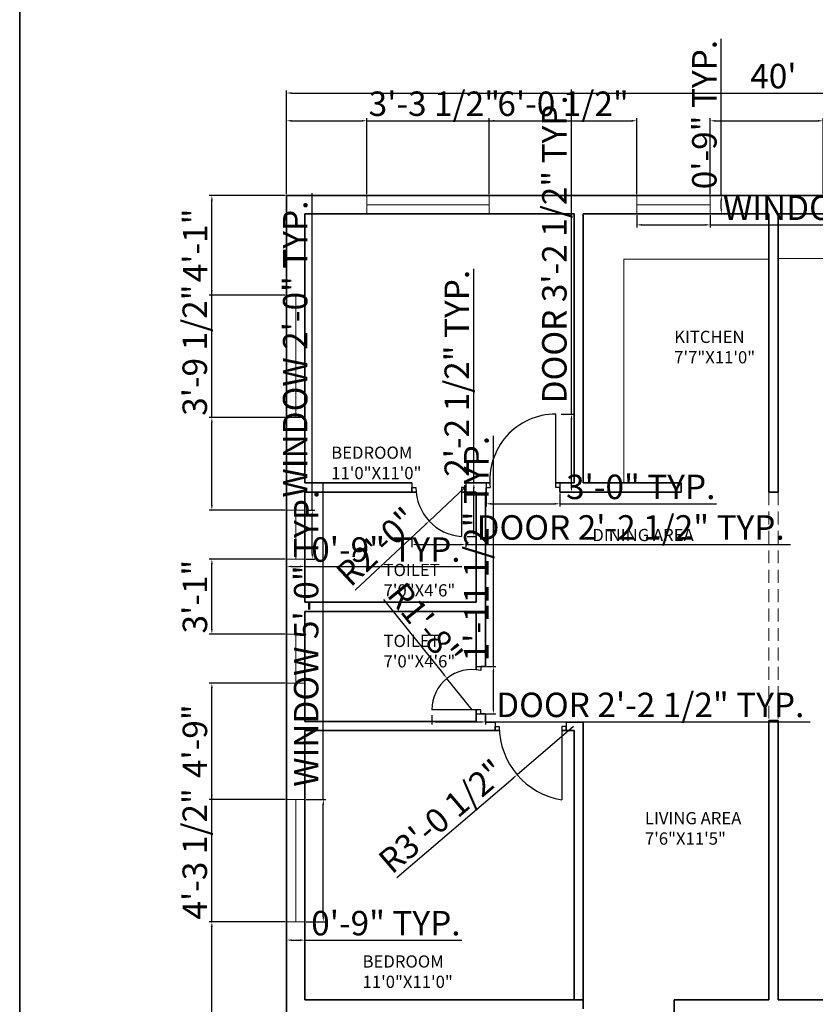
# Model space of a CAD drawing. Units: inches. Extents: x 2142 to 3604, y 1690 to 2981.
# Tile 2 of 9: x 2142 to 2532, y 2019 to 2502. Entities that reach past the tile are written whole.
import ezdxf

# ---------------------------------------------------------------- set-up
doc = ezdxf.new("R2010")
doc.units = ezdxf.units.IN
doc.linetypes.add('DASHED2', pattern=[9.525, 6.35, -3.175])
for name, color, linetype, lineweight in [('A-ANNO-DIMS', 2, 'Continuous', 18), ('A-ANNO-TTLB', 7, 'Continuous', 35), ('A-AREA-IDEN', 7, 'Continuous', 18), ('A-DOOR', 4, 'Continuous', 25), ('A-FLOR-FIXT', 8, 'Continuous', 18), ('A-GLAZ', 4, 'Continuous', 18), ('A-WALL', 7, 'Continuous', 35), ('A-WALL-OVHD', 254, 'DASHED2', 18)]:
    doc.layers.add(name, color=color, linetype=linetype, lineweight=lineweight)
doc.styles.get("Standard").update_dxf_attribs({"font": 'arial.ttf'})
doc.dimstyles.new('ISO-25', dxfattribs={"dimtxt": 12, "dimasz": 2.5, "dimexe": 1.25, "dimexo": 0.625, "dimtad": 1, "dimdec": 0, "dimlunit": 3, "dimtxsty": 'Standard', "dimcen": 2.5, "dimadec": 0, "dimazin": 0, "dimtfac": 1, "dimtdec": 0, "dimtmove": 0, "dimatfit": 3, "dimfxl": 1, "dimarcsym": 0})

# ---------------------------------------------------------------- blocks, each defined once
blk = doc.blocks.new('*D1')
at = {"layer": 'A-ANNO-DIMS', "color": 0, "lineweight": -2, "transparency": 16777216}
for p, q in [((2272.99, 2416.32), (2272.99, 2467.23)), ((2275.49, 2465.98), (2747.99, 2465.98)), ((2750.49, 2416.32), (2750.49, 2467.23))]:
    blk.add_line(p, q, dxfattribs=at)
at = {"layer": 'A-ANNO-DIMS', "color": 0, "transparency": 16777216}
for points in [[(2275.49, 2466.4), (2275.49, 2465.56), (2272.99, 2465.98)], [(2747.99, 2466.4), (2747.99, 2465.56), (2750.49, 2465.98)]]:
    blk.add_solid(points, dxfattribs=at)
at = {"layer": 'Defpoints', "color": 0, "transparency": 16777216}
for p in [(2750.49, 2465.98), (2272.99, 2415.7), (2750.49, 2415.7)]:
    blk.add_point(p, dxfattribs=at)
at = {"layer": 'A-ANNO-DIMS', "color": 0, "transparency": 16777216, "insert": (2511.74, 2472.73), "char_height": 12, "attachment_point": 5}
blk.add_mtext("40'", dxfattribs=at)
blk = doc.blocks.new('DOOR-BED-REAR-L')
for p, q in [((34.09, 2.25), (34.09, 38.25)), ((0, 4.5), (0, 0)), ((0, 0), (0, 2.25)), ((0, 2.25), (2, 2.25)), ((36.09, 2.25), (34.09, 2.25)), ((36.09, 4.5), (36.09, 0)), ((36.09, 0), (36.09, 2.25))]:
    blk.add_line(p, q)
blk.add_arc((34.09, 5.95), 32.3, 90, 186.5737)
blk = doc.blocks.new('DOOR-BATH-REAR-L')
for p, q in [((0, 26.25), (0, 21.75)), ((26.43, 26.25), (26.43, 21.75)), ((0, 21.75), (0, 24)), ((0, 24), (2, 24)), ((26.43, 24), (24.43, 24)), ((24.43, 24), (24.43, 0)), ((26.43, 21.75), (26.43, 24))]:
    blk.add_line(p, q)
blk.add_arc((26.05, 24), 24.05, 180, 266.1376)
blk = doc.blocks.new('DOOR-BATH-FRONT-L')
for p, q in [((21.75, 23.31), (26.25, 23.31)), ((26.25, 23.31), (24, 23.31)), ((24, 23.31), (24, 21.31)), ((24, 2), (0, 2)), ((24, 0), (24, 2)), ((21.75, 0), (26.25, 0)), ((26.25, 0), (24, 0))]:
    blk.add_line(p, q)
blk.add_arc((19.77, 2), 19.77, 77.6385, 180)
blk = doc.blocks.new('DOOR-BED-MID-L')
for p, q in [((0, 38.05), (0, 33.95)), ((0, 33.95), (0, 36)), ((0, 36), (2, 36)), ((34.72, 36), (32.72, 36)), ((32.72, 36), (32.72, 0)), ((34.72, 38.05), (34.72, 38.05)), ((34.72, 38.05), (34.72, 33.95)), ((34.72, 33.95), (34.72, 36))]:
    blk.add_line(p, q)
blk.add_arc((38.45, 36), 36.45, 180, 260.9442)
blk = doc.blocks.new('COUNTER-KITCHEN-L')
for p, q in [((0, 0), (0, 109.77)), ((0, 109.77), (71.11, 109.77))]:
    blk.add_line(p, q)
blk = doc.blocks.new('COUNTER-KITCHEN-R')
for p, q in [((0, 110.14), (69.54, 110.14)), ((69.54, 110.14), (69.54, 0))]:
    blk.add_line(p, q)
blk = doc.blocks.new('WINDOW-60')
for p, q in [((0, 60), (9, 60)), ((9, 60), (4.5, 60)), ((4.5, 60), (4.5, 0)), ((4.5, 0), (0, 0)), ((0, 0), (9, 0))]:
    blk.add_line(p, q)
blk = doc.blocks.new('WINDOW-24')
for p, q in [((0, 24), (9, 24)), ((9, 24), (4.5, 24)), ((4.5, 24), (4.5, 0)), ((4.5, 0), (0, 0)), ((0, 0), (9, 0))]:
    blk.add_line(p, q)
blk = doc.blocks.new('WINDOW-36')
for p, q in [((0, 9), (0, 0)), ((36, 4.5), (36, 9)), ((36, 9), (36, 0)), ((0, 0), (0, 4.5)), ((0, 4.5), (36, 4.5))]:
    blk.add_line(p, q)
blk = doc.blocks.new('WINDOW-60-B')
for p, q in [((4.5, 60), (0, 60)), ((0, 60), (9, 60)), ((4.5, 0), (4.5, 60)), ((9, 0), (0, 0)), ((0, 0), (4.5, 0))]:
    blk.add_line(p, q)
blk = doc.blocks.new('*D29')
at = {"layer": 'A-ANNO-DIMS', "color": 0, "lineweight": -2, "transparency": 16777216}
for p, q in [((2290.99, 2119.45), (2290.99, 2275.05)), ((2282.61, 2119.45), (2292.24, 2119.45)), ((2290.99, 2061.95), (2290.99, 2116.95)), ((2282.61, 2059.45), (2292.24, 2059.45))]:
    blk.add_line(p, q, dxfattribs=at)
at = {"layer": 'A-ANNO-DIMS', "color": 0, "transparency": 16777216}
for points in [[(2290.57, 2116.95), (2291.4, 2116.95), (2290.99, 2119.45)], [(2290.57, 2061.95), (2291.4, 2061.95), (2290.99, 2059.45)]]:
    blk.add_solid(points, dxfattribs=at)
at = {"layer": 'Defpoints', "color": 0, "transparency": 16777216}
for p in [(2281.99, 2119.45), (2290.99, 2119.45), (2281.99, 2059.45)]:
    blk.add_point(p, dxfattribs=at)
at = {"layer": 'A-ANNO-DIMS', "color": 0, "transparency": 16777216, "insert": (2284.15, 2198.5), "char_height": 12, "attachment_point": 5, "rotation": 90}
blk.add_mtext('WINDOW 5\'-0" TYP.', dxfattribs=at)
blk = doc.blocks.new('*D30')
at = {"layer": 'A-ANNO-DIMS', "color": 0, "lineweight": -2, "transparency": 16777216}
for p, q in [((2272.99, 2058.82), (2272.99, 2049.2)), ((2281.99, 2058.82), (2281.99, 2049.2)), ((2275.49, 2050.45), (2279.49, 2050.45)), ((2281.99, 2050.45), (2358.88, 2050.45))]:
    blk.add_line(p, q, dxfattribs=at)
at = {"layer": 'A-ANNO-DIMS', "color": 0, "transparency": 16777216}
for points in [[(2275.49, 2050.86), (2275.49, 2050.03), (2272.99, 2050.45)], [(2279.49, 2050.86), (2279.49, 2050.03), (2281.99, 2050.45)]]:
    blk.add_solid(points, dxfattribs=at)
at = {"layer": 'Defpoints', "color": 0, "transparency": 16777216}
for p in [(2272.99, 2059.45), (2281.99, 2059.45), (2281.99, 2050.45)]:
    blk.add_point(p, dxfattribs=at)
at = {"layer": 'A-ANNO-DIMS', "color": 0, "transparency": 16777216, "insert": (2321.68, 2057.2), "char_height": 12, "attachment_point": 5}
blk.add_mtext('0\'-9" TYP.', dxfattribs=at)
blk = doc.blocks.new('*D31')
at = {"layer": 'A-ANNO-DIMS', "color": 0, "lineweight": -2, "transparency": 16777216}
for p, q in [((2285.59, 2261.33), (2285.59, 2416.93)), ((2282.61, 2261.33), (2286.84, 2261.33)), ((2285.59, 2239.83), (2285.59, 2258.83)), ((2282.61, 2237.33), (2286.84, 2237.33))]:
    blk.add_line(p, q, dxfattribs=at)
at = {"layer": 'A-ANNO-DIMS', "color": 0, "transparency": 16777216}
for points in [[(2285.17, 2258.83), (2286, 2258.83), (2285.59, 2261.33)], [(2285.17, 2239.83), (2286, 2239.83), (2285.59, 2237.33)]]:
    blk.add_solid(points, dxfattribs=at)
at = {"layer": 'Defpoints', "color": 0, "transparency": 16777216}
for p in [(2281.99, 2261.33), (2285.59, 2261.33), (2281.99, 2237.33)]:
    blk.add_point(p, dxfattribs=at)
at = {"layer": 'A-ANNO-DIMS', "color": 0, "transparency": 16777216, "insert": (2278.75, 2340.38), "char_height": 12, "attachment_point": 5, "rotation": 90}
blk.add_mtext('WINDOW 2\'-0" TYP.', dxfattribs=at)
blk = doc.blocks.new('*D32')
at = {"layer": 'A-ANNO-DIMS', "color": 0, "lineweight": -2, "transparency": 16777216}
for p, q in [((2272.99, 2236.7), (2272.99, 2232.48)), ((2281.99, 2236.7), (2281.99, 2232.48)), ((2275.49, 2233.73), (2279.49, 2233.73)), ((2281.99, 2233.73), (2358.88, 2233.73))]:
    blk.add_line(p, q, dxfattribs=at)
at = {"layer": 'A-ANNO-DIMS', "color": 0, "transparency": 16777216}
for points in [[(2275.49, 2234.15), (2275.49, 2233.31), (2272.99, 2233.73)], [(2279.49, 2234.15), (2279.49, 2233.31), (2281.99, 2233.73)]]:
    blk.add_solid(points, dxfattribs=at)
at = {"layer": 'Defpoints', "color": 0, "transparency": 16777216}
for p in [(2272.99, 2237.33), (2281.99, 2237.33), (2281.99, 2233.73)]:
    blk.add_point(p, dxfattribs=at)
at = {"layer": 'A-ANNO-DIMS', "color": 0, "transparency": 16777216, "insert": (2321.68, 2240.48), "char_height": 12, "attachment_point": 5}
blk.add_mtext('0\'-9" TYP.', dxfattribs=at)
blk = doc.blocks.new('*D33')
at = {"layer": 'A-ANNO-DIMS', "color": 0, "lineweight": -2, "transparency": 16777216}
for p, q in [((2444.78, 2406.07), (2444.78, 2400.05)), ((2480.78, 2406.07), (2480.78, 2400.05)), ((2447.28, 2401.3), (2478.28, 2401.3)), ((2480.78, 2401.3), (2636.38, 2401.3))]:
    blk.add_line(p, q, dxfattribs=at)
at = {"layer": 'A-ANNO-DIMS', "color": 0, "transparency": 16777216}
for points in [[(2447.28, 2401.71), (2447.28, 2400.88), (2444.78, 2401.3)], [(2478.28, 2401.71), (2478.28, 2400.88), (2480.78, 2401.3)]]:
    blk.add_solid(points, dxfattribs=at)
at = {"layer": 'Defpoints', "color": 0, "transparency": 16777216}
for p in [(2444.78, 2406.7), (2480.78, 2406.7), (2480.78, 2401.3)]:
    blk.add_point(p, dxfattribs=at)
at = {"layer": 'A-ANNO-DIMS', "color": 0, "transparency": 16777216, "insert": (2559.83, 2408.13), "char_height": 12, "attachment_point": 5}
blk.add_mtext('WINDOW 3\'-0" TYP.', dxfattribs=at)
blk = doc.blocks.new('*D34')
at = {"layer": 'A-ANNO-DIMS', "color": 0, "lineweight": -2, "transparency": 16777216}
for p, q in [((2486.18, 2415.7), (2486.18, 2492.59)), ((2481.4, 2415.7), (2487.43, 2415.7)), ((2486.18, 2409.2), (2486.18, 2413.2)), ((2481.4, 2406.7), (2487.43, 2406.7))]:
    blk.add_line(p, q, dxfattribs=at)
at = {"layer": 'A-ANNO-DIMS', "color": 0, "transparency": 16777216}
for points in [[(2485.76, 2413.2), (2486.59, 2413.2), (2486.18, 2415.7)], [(2485.76, 2409.2), (2486.59, 2409.2), (2486.18, 2406.7)]]:
    blk.add_solid(points, dxfattribs=at)
at = {"layer": 'Defpoints', "color": 0, "transparency": 16777216}
for p in [(2480.78, 2415.7), (2486.18, 2415.7), (2480.78, 2406.7)]:
    blk.add_point(p, dxfattribs=at)
at = {"layer": 'A-ANNO-DIMS', "color": 0, "transparency": 16777216, "insert": (2479.42, 2455.39), "char_height": 12, "attachment_point": 5, "rotation": 90}
blk.add_mtext('0\'-9" TYP.', dxfattribs=at)
blk = doc.blocks.new('*D43')
at = {"layer": 'A-ANNO-DIMS', "color": 0, "lineweight": -2, "transparency": 16777216}
for p, q in [((2412.71, 2308.45), (2412.71, 2467.66)), ((2407.6, 2308.45), (2413.96, 2308.45)), ((2412.71, 2272.7), (2412.71, 2305.95)), ((2407.6, 2270.2), (2413.96, 2270.2))]:
    blk.add_line(p, q, dxfattribs=at)
at = {"layer": 'A-ANNO-DIMS', "color": 0, "transparency": 16777216}
for points in [[(2412.29, 2305.95), (2413.13, 2305.95), (2412.71, 2308.45)], [(2412.29, 2272.7), (2413.13, 2272.7), (2412.71, 2270.2)]]:
    blk.add_solid(points, dxfattribs=at)
at = {"layer": 'Defpoints', "color": 0, "transparency": 16777216}
for p in [(2406.97, 2308.45), (2412.71, 2308.45), (2406.97, 2270.2)]:
    blk.add_point(p, dxfattribs=at)
at = {"layer": 'A-ANNO-DIMS', "color": 0, "transparency": 16777216, "insert": (2405.87, 2389.3), "char_height": 12, "attachment_point": 5, "rotation": 90}
blk.add_mtext('DOOR 3\'-2 1/2" TYP.', dxfattribs=at)
blk = doc.blocks.new('*D44')
at = {"layer": 'A-ANNO-DIMS', "color": 0, "lineweight": -2, "transparency": 16777216}
for p, q in [((2370.88, 2269.57), (2370.88, 2263.21)), ((2406.97, 2269.57), (2406.97, 2263.21)), ((2373.38, 2264.46), (2404.47, 2264.46)), ((2406.97, 2264.46), (2483.86, 2264.46))]:
    blk.add_line(p, q, dxfattribs=at)
at = {"layer": 'A-ANNO-DIMS', "color": 0, "transparency": 16777216}
for points in [[(2373.38, 2264.88), (2373.38, 2264.04), (2370.88, 2264.46)], [(2404.47, 2264.88), (2404.47, 2264.04), (2406.97, 2264.46)]]:
    blk.add_solid(points, dxfattribs=at)
at = {"layer": 'Defpoints', "color": 0, "transparency": 16777216}
for p in [(2370.88, 2270.2), (2406.97, 2270.2), (2406.97, 2264.46)]:
    blk.add_point(p, dxfattribs=at)
at = {"layer": 'A-ANNO-DIMS', "color": 0, "transparency": 16777216, "insert": (2446.67, 2271.22), "char_height": 12, "attachment_point": 5}
blk.add_mtext('3\'-0" TYP.', dxfattribs=at)
blk = doc.blocks.new('*D47')
at = {"layer": 'A-ANNO-DIMS', "color": 0, "lineweight": -2, "transparency": 16777216}
for p, q in [((2334.42, 2247.82), (2334.42, 2243.23)), ((2360.85, 2247.82), (2360.85, 2243.23)), ((2336.92, 2244.48), (2358.35, 2244.48)), ((2360.85, 2244.48), (2520.06, 2244.48))]:
    blk.add_line(p, q, dxfattribs=at)
at = {"layer": 'A-ANNO-DIMS', "color": 0, "transparency": 16777216}
for points in [[(2336.92, 2244.9), (2336.92, 2244.06), (2334.42, 2244.48)], [(2358.35, 2244.9), (2358.35, 2244.06), (2360.85, 2244.48)]]:
    blk.add_solid(points, dxfattribs=at)
at = {"layer": 'Defpoints', "color": 0, "transparency": 16777216}
for p in [(2334.42, 2248.45), (2360.85, 2248.45), (2360.85, 2244.48)]:
    blk.add_point(p, dxfattribs=at)
at = {"layer": 'A-ANNO-DIMS', "color": 0, "transparency": 16777216, "insert": (2441.71, 2251.32), "char_height": 12, "attachment_point": 5}
blk.add_mtext('DOOR 2\'-2 1/2" TYP.', dxfattribs=at)
blk = doc.blocks.new('*D48')
at = {"layer": 'A-ANNO-DIMS', "color": 0, "lineweight": -2, "transparency": 16777216}
for p, q in [((2364.82, 2274.7), (2364.82, 2379.76)), ((2361.48, 2274.7), (2366.07, 2274.7)), ((2364.82, 2250.95), (2364.82, 2272.2)), ((2361.48, 2248.45), (2366.07, 2248.45))]:
    blk.add_line(p, q, dxfattribs=at)
at = {"layer": 'A-ANNO-DIMS', "color": 0, "transparency": 16777216}
for points in [[(2364.4, 2272.2), (2365.24, 2272.2), (2364.82, 2274.7)], [(2364.4, 2250.95), (2365.24, 2250.95), (2364.82, 2248.45)]]:
    blk.add_solid(points, dxfattribs=at)
at = {"layer": 'Defpoints', "color": 0, "transparency": 16777216}
for p in [(2360.85, 2274.7), (2364.82, 2274.7), (2360.85, 2248.45)]:
    blk.add_point(p, dxfattribs=at)
at = {"layer": 'A-ANNO-DIMS', "color": 0, "transparency": 16777216, "insert": (2357.99, 2328.48), "char_height": 12, "attachment_point": 5, "rotation": 90}
blk.add_mtext('2\'-2 1/2" TYP.', dxfattribs=at)
blk = doc.blocks.new('*D51')
at = {"layer": 'A-ANNO-DIMS', "color": 0, "lineweight": -2, "transparency": 16777216}
for p, q in [((2344.24, 2160.76), (2344.24, 2156.2)), ((2370.49, 2160.76), (2370.49, 2156.2)), ((2346.74, 2157.45), (2367.99, 2157.45)), ((2370.49, 2157.45), (2529.7, 2157.45))]:
    blk.add_line(p, q, dxfattribs=at)
at = {"layer": 'A-ANNO-DIMS', "color": 0, "transparency": 16777216}
for points in [[(2346.74, 2157.87), (2346.74, 2157.03), (2344.24, 2157.45)], [(2367.99, 2157.87), (2367.99, 2157.03), (2370.49, 2157.45)]]:
    blk.add_solid(points, dxfattribs=at)
at = {"layer": 'Defpoints', "color": 0, "transparency": 16777216}
for p in [(2344.24, 2161.39), (2370.49, 2161.39), (2370.49, 2157.45)]:
    blk.add_point(p, dxfattribs=at)
at = {"layer": 'A-ANNO-DIMS', "color": 0, "transparency": 16777216, "insert": (2451.34, 2164.28), "char_height": 12, "attachment_point": 5}
blk.add_mtext('DOOR 2\'-2 1/2" TYP.', dxfattribs=at)
blk = doc.blocks.new('*D52')
at = {"layer": 'A-ANNO-DIMS', "color": 0, "lineweight": -2, "transparency": 16777216}
for p, q in [((2374.42, 2184.7), (2374.42, 2297.75)), ((2371.11, 2184.7), (2375.67, 2184.7)), ((2374.42, 2163.89), (2374.42, 2182.2)), ((2371.11, 2161.39), (2375.67, 2161.39))]:
    blk.add_line(p, q, dxfattribs=at)
at = {"layer": 'A-ANNO-DIMS', "color": 0, "transparency": 16777216}
for points in [[(2374.01, 2182.2), (2374.84, 2182.2), (2374.42, 2184.7)], [(2374.01, 2163.89), (2374.84, 2163.89), (2374.42, 2161.39)]]:
    blk.add_solid(points, dxfattribs=at)
at = {"layer": 'Defpoints', "color": 0, "transparency": 16777216}
for p in [(2370.49, 2184.7), (2374.42, 2184.7), (2370.49, 2161.39)]:
    blk.add_point(p, dxfattribs=at)
at = {"layer": 'A-ANNO-DIMS', "color": 0, "transparency": 16777216, "insert": (2367.59, 2242.47), "char_height": 12, "attachment_point": 5, "rotation": 90}
blk.add_mtext('1\'-11 1/2" TYP.', dxfattribs=at)
blk = doc.blocks.new('*D100')
at = {"layer": 'A-ANNO-DIMS', "color": 0, "lineweight": -2, "transparency": 16777216}
for p, q in [((2236.34, 2059.45), (2236.34, 2123.54)), ((2272.36, 2059.45), (2235.09, 2059.45)), ((2236.34, 2010.33), (2236.34, 2056.95)), ((2272.36, 2007.83), (2235.09, 2007.83))]:
    blk.add_line(p, q, dxfattribs=at)
at = {"layer": 'A-ANNO-DIMS', "color": 0, "transparency": 16777216}
for points in [[(2235.92, 2056.95), (2236.75, 2056.95), (2236.34, 2059.45)], [(2235.92, 2010.33), (2236.75, 2010.33), (2236.34, 2007.83)]]:
    blk.add_solid(points, dxfattribs=at)
at = {"layer": 'Defpoints', "color": 0, "transparency": 16777216}
for p in [(2236.34, 2059.45), (2272.99, 2059.45), (2272.99, 2007.83)]:
    blk.add_point(p, dxfattribs=at)
at = {"layer": 'A-ANNO-DIMS', "color": 0, "transparency": 16777216, "insert": (2229.5, 2092.74), "char_height": 12, "attachment_point": 5, "rotation": 90}
blk.add_mtext('4\'-3 1/2"', dxfattribs=at)
blk = doc.blocks.new('*D101')
at = {"layer": 'A-ANNO-DIMS', "color": 0, "lineweight": -2, "transparency": 16777216}
for p, q in [((2272.36, 2176.55), (2235.09, 2176.55)), ((2236.34, 2121.95), (2236.34, 2174.05)), ((2272.36, 2119.45), (2235.09, 2119.45))]:
    blk.add_line(p, q, dxfattribs=at)
at = {"layer": 'A-ANNO-DIMS', "color": 0, "transparency": 16777216}
for points in [[(2235.92, 2174.05), (2236.75, 2174.05), (2236.34, 2176.55)], [(2235.92, 2121.95), (2236.75, 2121.95), (2236.34, 2119.45)]]:
    blk.add_solid(points, dxfattribs=at)
at = {"layer": 'Defpoints', "color": 0, "transparency": 16777216}
for p in [(2236.34, 2176.55), (2272.99, 2176.55), (2272.99, 2119.45)]:
    blk.add_point(p, dxfattribs=at)
at = {"layer": 'A-ANNO-DIMS', "color": 0, "transparency": 16777216, "insert": (2229.58, 2148), "char_height": 12, "attachment_point": 5, "rotation": 90}
blk.add_mtext('4\'-9"', dxfattribs=at)
blk = doc.blocks.new('*D102')
at = {"layer": 'A-ANNO-DIMS', "color": 0, "lineweight": -2, "transparency": 16777216}
for p, q in [((2272.36, 2237.33), (2235.09, 2237.33)), ((2236.34, 2203.05), (2236.34, 2234.83)), ((2272.36, 2200.55), (2235.09, 2200.55))]:
    blk.add_line(p, q, dxfattribs=at)
at = {"layer": 'A-ANNO-DIMS', "color": 0, "transparency": 16777216}
for points in [[(2235.92, 2234.83), (2236.75, 2234.83), (2236.34, 2237.33)], [(2235.92, 2203.05), (2236.75, 2203.05), (2236.34, 2200.55)]]:
    blk.add_solid(points, dxfattribs=at)
at = {"layer": 'Defpoints', "color": 0, "transparency": 16777216}
for p in [(2236.34, 2237.33), (2272.99, 2237.33), (2272.99, 2200.55)]:
    blk.add_point(p, dxfattribs=at)
at = {"layer": 'A-ANNO-DIMS', "color": 0, "transparency": 16777216, "insert": (2229.58, 2218.94), "char_height": 12, "attachment_point": 5, "rotation": 90}
blk.add_mtext('3\'-1"', dxfattribs=at)
blk = doc.blocks.new('*D103')
at = {"layer": 'A-ANNO-DIMS', "color": 0, "lineweight": -2, "transparency": 16777216}
for p, q in [((2236.34, 2306.79), (2236.34, 2370.39)), ((2272.36, 2306.79), (2235.09, 2306.79)), ((2236.34, 2263.83), (2236.34, 2304.29)), ((2272.36, 2261.33), (2235.09, 2261.33))]:
    blk.add_line(p, q, dxfattribs=at)
at = {"layer": 'A-ANNO-DIMS', "color": 0, "transparency": 16777216}
for points in [[(2235.92, 2304.29), (2236.75, 2304.29), (2236.34, 2306.79)], [(2235.92, 2263.83), (2236.75, 2263.83), (2236.34, 2261.33)]]:
    blk.add_solid(points, dxfattribs=at)
at = {"layer": 'Defpoints', "color": 0, "transparency": 16777216}
for p in [(2236.34, 2306.79), (2272.99, 2306.79), (2272.99, 2261.33)]:
    blk.add_point(p, dxfattribs=at)
at = {"layer": 'A-ANNO-DIMS', "color": 0, "transparency": 16777216, "insert": (2229.5, 2339.84), "char_height": 12, "attachment_point": 5, "rotation": 90}
blk.add_mtext('3\'-9 1/2"', dxfattribs=at)
blk = doc.blocks.new('*D104')
at = {"layer": 'A-ANNO-DIMS', "color": 0, "lineweight": -2, "transparency": 16777216}
for p, q in [((2272.36, 2415.7), (2235.09, 2415.7)), ((2236.34, 2369.29), (2236.34, 2413.2)), ((2272.36, 2366.79), (2235.09, 2366.79))]:
    blk.add_line(p, q, dxfattribs=at)
at = {"layer": 'A-ANNO-DIMS', "color": 0, "transparency": 16777216}
for points in [[(2235.92, 2413.2), (2236.75, 2413.2), (2236.34, 2415.7)], [(2235.92, 2369.29), (2236.75, 2369.29), (2236.34, 2366.79)]]:
    blk.add_solid(points, dxfattribs=at)
at = {"layer": 'Defpoints', "color": 0, "transparency": 16777216}
for p in [(2236.34, 2415.7), (2272.99, 2415.7), (2272.99, 2366.79)]:
    blk.add_point(p, dxfattribs=at)
at = {"layer": 'A-ANNO-DIMS', "color": 0, "transparency": 16777216, "insert": (2229.69, 2391.24), "char_height": 12, "attachment_point": 5, "rotation": 90}
blk.add_mtext('4\'-1"', dxfattribs=at)
blk = doc.blocks.new('*D105')
at = {"layer": 'A-ANNO-DIMS', "color": 0, "lineweight": -2, "transparency": 16777216}
for p, q in [((2272.99, 2416.32), (2272.99, 2453.6)), ((2275.49, 2452.35), (2309.89, 2452.35)), ((2312.39, 2416.32), (2312.39, 2453.6)), ((2312.39, 2452.35), (2375.99, 2452.35))]:
    blk.add_line(p, q, dxfattribs=at)
at = {"layer": 'A-ANNO-DIMS', "color": 0, "transparency": 16777216}
for points in [[(2275.49, 2452.76), (2275.49, 2451.93), (2272.99, 2452.35)], [(2309.89, 2452.76), (2309.89, 2451.93), (2312.39, 2452.35)]]:
    blk.add_solid(points, dxfattribs=at)
at = {"layer": 'Defpoints', "color": 0, "transparency": 16777216}
for p in [(2312.39, 2452.35), (2272.99, 2415.7), (2312.39, 2415.7)]:
    blk.add_point(p, dxfattribs=at)
at = {"layer": 'A-ANNO-DIMS', "color": 0, "transparency": 16777216, "insert": (2345.44, 2459.18), "char_height": 12, "attachment_point": 5}
blk.add_mtext('3\'-3 1/2"', dxfattribs=at)
blk = doc.blocks.new('*D106')
at = {"layer": 'A-ANNO-DIMS', "color": 0, "lineweight": -2, "transparency": 16777216}
for p, q in [((2372.39, 2416.32), (2372.39, 2453.6)), ((2374.89, 2452.35), (2442.28, 2452.35)), ((2444.78, 2416.32), (2444.78, 2453.6))]:
    blk.add_line(p, q, dxfattribs=at)
at = {"layer": 'A-ANNO-DIMS', "color": 0, "transparency": 16777216}
for points in [[(2374.89, 2452.76), (2374.89, 2451.93), (2372.39, 2452.35)], [(2442.28, 2452.76), (2442.28, 2451.93), (2444.78, 2452.35)]]:
    blk.add_solid(points, dxfattribs=at)
at = {"layer": 'Defpoints', "color": 0, "transparency": 16777216}
for p in [(2444.78, 2452.35), (2372.39, 2415.7), (2444.78, 2415.7)]:
    blk.add_point(p, dxfattribs=at)
at = {"layer": 'A-ANNO-DIMS', "color": 0, "transparency": 16777216, "insert": (2408.58, 2459.18), "char_height": 12, "attachment_point": 5}
blk.add_mtext('6\'-0 1/2"', dxfattribs=at)
blk = doc.blocks.new('*D107')
at = {"layer": 'A-ANNO-DIMS', "color": 0, "lineweight": -2, "transparency": 16777216}
for p, q in [((2480.78, 2416.32), (2480.78, 2453.6)), ((2483.28, 2452.35), (2533.61, 2452.35)), ((2536.11, 2416.32), (2536.11, 2453.6)), ((2536.11, 2452.35), (2600.21, 2452.35))]:
    blk.add_line(p, q, dxfattribs=at)
at = {"layer": 'A-ANNO-DIMS', "color": 0, "transparency": 16777216}
for points in [[(2483.28, 2452.76), (2483.28, 2451.93), (2480.78, 2452.35)], [(2533.61, 2452.76), (2533.61, 2451.93), (2536.11, 2452.35)]]:
    blk.add_solid(points, dxfattribs=at)
at = {"layer": 'Defpoints', "color": 0, "transparency": 16777216}
for p in [(2536.11, 2452.35), (2480.78, 2415.7), (2536.11, 2415.7)]:
    blk.add_point(p, dxfattribs=at)
at = {"layer": 'A-ANNO-DIMS', "color": 0, "transparency": 16777216, "insert": (2569.41, 2459.18), "char_height": 12, "attachment_point": 5}
blk.add_mtext('4\'-7 1/2"', dxfattribs=at)
blk = doc.blocks.new('*D123')
at = {"layer": 'A-ANNO-DIMS', "color": 0, "lineweight": -2, "transparency": 16777216}
for p, q in [((2413.77, 2155.24), (2386.03, 2131.58)), ((2327.01, 2081.22), (2384.13, 2129.96))]:
    blk.add_line(p, q, dxfattribs=at)
at = {"layer": 'A-ANNO-DIMS', "color": 0, "transparency": 16777216}
blk.add_solid([(2383.86, 2130.28), (2384.4, 2129.64), (2386.03, 2131.58)], dxfattribs=at)
at = {"layer": 'Defpoints', "color": 0, "transparency": 16777216}
for p in [(2413.77, 2155.24), (2386.03, 2131.58)]:
    blk.add_point(p, dxfattribs=at)
at = {"layer": 'A-ANNO-DIMS', "color": 0, "transparency": 16777216, "insert": (2350.18, 2109.98), "char_height": 12, "attachment_point": 5, "rotation": 40.4718}
blk.add_mtext('R3\'-0 1/2"', dxfattribs=at)
blk = doc.blocks.new('*D131')
at = {"layer": 'A-ANNO-DIMS', "color": 0, "lineweight": -2, "transparency": 16777216}
for p, q in [((2360.47, 2272.45), (2342.9, 2256.02)), ((2306.64, 2222.13), (2341.07, 2254.31))]:
    blk.add_line(p, q, dxfattribs=at)
at = {"layer": 'A-ANNO-DIMS', "color": 0, "transparency": 16777216}
blk.add_solid([(2340.79, 2254.62), (2341.36, 2254.01), (2342.9, 2256.02)], dxfattribs=at)
at = {"layer": 'Defpoints', "color": 0, "transparency": 16777216}
for p in [(2360.47, 2272.45), (2342.9, 2256.02)]:
    blk.add_point(p, dxfattribs=at)
at = {"layer": 'A-ANNO-DIMS', "color": 0, "transparency": 16777216, "insert": (2318.33, 2242.3), "char_height": 12, "attachment_point": 5, "rotation": 43.0693}
blk.add_mtext('R2\'-0"', dxfattribs=at)
blk = doc.blocks.new('*D135')
at = {"layer": 'A-ANNO-DIMS', "color": 0, "lineweight": -2, "transparency": 16777216}
for p, q in [((2320.5, 2217.46), (2350.05, 2180.74)), ((2364, 2163.39), (2351.61, 2178.79))]:
    blk.add_line(p, q, dxfattribs=at)
at = {"layer": 'A-ANNO-DIMS', "color": 0, "transparency": 16777216}
blk.add_solid([(2350.37, 2181), (2349.72, 2180.48), (2351.61, 2178.79)], dxfattribs=at)
at = {"layer": 'Defpoints', "color": 0, "transparency": 16777216}
for p in [(2351.61, 2178.79), (2364, 2163.39)]:
    blk.add_point(p, dxfattribs=at)
at = {"layer": 'A-ANNO-DIMS', "color": 0, "transparency": 16777216, "insert": (2339.75, 2204.3), "char_height": 12, "attachment_point": 5, "rotation": 308.8182}
blk.add_mtext('R1\'-8"', dxfattribs=at)

msp = doc.modelspace()

# ---------------------------------------------------------------- linework, layer by layer
at = {"layer": 'A-ANNO-TTLB'}
msp.add_lwpolyline([(2142.1, 2981.01), (3604.42, 2981.01), (3604.42, 1690.13), (2142.1, 1690.13)], close=True, dxfattribs=at)
at = {"layer": 'A-WALL'}
for p, q in [((2272.99, 2415.7), (2750.49, 2415.7)), ((2272.99, 2415.7), (2750.49, 2415.7)), ((2272.99, 2415.7), (2272.99, 1823.2)), ((2281.99, 2406.7), (2413.99, 2406.7)), ((2281.99, 2406.7), (2281.99, 2274.7)), ((2413.99, 2406.7), (2413.99, 2274.7)), ((2418.49, 2406.7), (2418.49, 2274.7)), ((2418.49, 2406.7), (2509.49, 2406.7)), ((2509.49, 2406.7), (2509.49, 2270.2)), ((2513.99, 2406.7), (2513.99, 2270.2)), ((2513.99, 2406.7), (2604.99, 2406.7)), ((2281.99, 2274.7), (2334.42, 2274.7)), ((2281.99, 2270.2), (2336.52, 2270.2)), ((2281.99, 2270.2), (2281.99, 2216.2)), ((2358.85, 2270.2), (2365.99, 2270.2)), ((2360.85, 2274.7), (2372.7, 2274.7)), ((2365.99, 2216.2), (2365.99, 2270.2)), ((2370.49, 2270.2), (2370.49, 2184.7)), ((2370.49, 2270.2), (2370.88, 2270.2)), ((2404.97, 2274.7), (2413.99, 2274.7)), ((2406.97, 2270.2), (2466.52, 2270.2)), ((2418.49, 2274.7), (2466.52, 2274.7)), ((2466.52, 2274.7), (2466.52, 2270.2)), ((2509.49, 2270.2), (2513.99, 2270.2)), ((2281.99, 2216.2), (2365.99, 2216.2)), ((2281.99, 2211.7), (2365.99, 2211.7)), ((2281.99, 2211.7), (2281.99, 2157.7)), ((2365.99, 2183.06), (2365.99, 2211.7)), ((2365.99, 2157.7), (2365.99, 2163.39)), ((2370.49, 2161.39), (2370.49, 2157.29)), ((2281.99, 2157.7), (2365.99, 2157.7)), ((2370.49, 2157.29), (2375.31, 2157.29)), ((2410.03, 2157.29), (2418.49, 2157.29)), ((2418.49, 2157.29), (2418.49, 2016.7)), ((2513.99, 2158.2), (2509.49, 2158.2)), ((2509.49, 2158.2), (2509.49, 2021.2)), ((2513.99, 2021.2), (2513.99, 2158.2)), ((2513.99, 2158.2), (2513.99, 2021.2)), ((2281.99, 2153.2), (2370.49, 2153.2)), ((2281.99, 2153.2), (2365.99, 2153.2)), ((2281.99, 2153.2), (2281.99, 2021.2)), ((2370.49, 2153.2), (2377.37, 2153.2)), ((2408.03, 2153.2), (2413.99, 2153.2)), ((2413.99, 2153.2), (2413.99, 2021.2)), ((2281.99, 2021.2), (2418.49, 2021.2)), ((2462.99, 1884.7), (2462.99, 2021.2)), ((2509.49, 2021.2), (2462.99, 2021.2)), ((2560.49, 2021.2), (2513.99, 2021.2))]:
    msp.add_line(p, q, dxfattribs=at)
at = {"layer": 'A-WALL-OVHD'}
for p, q in [((2509.49, 2270.2), (2509.49, 2270.2)), ((2509.49, 2270.2), (2509.49, 2158.2)), ((2513.99, 2270.2), (2513.99, 2158.2))]:
    msp.add_line(p, q, dxfattribs=at)

# ---------------------------------------------------------------- block references
at = {"layer": 'A-DOOR'}
for name, p in [('DOOR-BED-REAR-L', (2370.88, 2270.2)), ('DOOR-BATH-REAR-L', (2334.42, 2248.45)), ('DOOR-BATH-FRONT-L', (2344.24, 2161.39)), ('DOOR-BED-MID-L', (2375.31, 2119.24))]:
    msp.add_blockref(name, p, dxfattribs=at)
at = {"layer": 'A-FLOR-FIXT'}
for name, p in [('COUNTER-KITCHEN-L', (2438.37, 2274.7)), ('COUNTER-KITCHEN-R', (2513.99, 2274.7))]:
    msp.add_blockref(name, p, dxfattribs=at)
at = {"layer": 'A-GLAZ', "extrusion": (0, 0, -1), "zscale": -1, "rotation": 270}
msp.add_blockref('WINDOW-60', (-2372.39, 2415.7), dxfattribs=at)
at = {"layer": 'A-GLAZ'}
for name, p in [('WINDOW-36', (2444.78, 2406.7)), ('WINDOW-60-B', (2272.99, 2306.79)), ('WINDOW-24', (2272.99, 2237.33)), ('WINDOW-24', (2272.99, 2176.55)), ('WINDOW-60', (2272.99, 2059.45))]:
    msp.add_blockref(name, p, dxfattribs=at)

# ---------------------------------------------------------------- texts
at = {"layer": 'A-AREA-IDEN', "char_height": 6, "attachment_point": 1}
for s, width, insert in [('KITCHEN\\P7\'7"X11\'0"', 106.5987, (2463.07, 2349.36)), ('BEDROOM\\P11\'0"X11\'0"', 75.5917, (2294.87, 2292.55)), ('DINING AREA', 86.5434, (2422.94, 2252.16)), ('TOILET\\P7\'0"X4\'6"', 54.861, (2320.54, 2235.01)), ('TOILET\\P7\'0"X4\'6"', 54.861, (2320.54, 2200.2)), ('LIVING AREA\\P7\'6"X11\'5" ', 119.5331, (2448.72, 2113.25)), ('BEDROOM\\P11\'0"X11\'0"', 121.5641, (2310.25, 2042.96))]:
    msp.add_mtext_dynamic_manual_height_columns(s, width=width, gutter_width=12.5, heights=[0], dxfattribs=dict(at, insert=insert))

# ---------------------------------------------------------------- dimensions: what is measured, and where the dimension line sits
at = {"layer": 'A-ANNO-DIMS'}
for base, p1, p2, text, picture, middle in [((2486.18, 2415.7), (2480.78, 2406.7), (2480.78, 2415.7), '<> TYP.', '*D34', (2479.42, 2455.39)), ((2412.71145544, 2308.44672184), (2406.97395544, 2270.19672184), (2406.97395544, 2308.44672184), 'DOOR <> TYP.', '*D43', (2405.87363143, 2389.30159906)), ((2285.59, 2261.33), (2281.99, 2237.33), (2281.99, 2261.33), 'WINDOW <> TYP.', '*D31', (2278.75, 2340.38)), ((2364.81867387, 2274.69672184), (2360.85352934, 2248.44672184), (2360.85352934, 2274.69672184), '<> TYP.', '*D48', (2357.98903539, 2328.47792921)), ((2374.42, 2184.7), (2370.49, 2161.39), (2370.49, 2184.7), '<> TYP.', '*D52', (2367.59, 2242.47)), ((2290.99, 2119.45), (2281.99, 2059.45), (2281.99, 2119.45), 'WINDOW <> TYP.', '*D29', (2284.15, 2198.5))]:
    dim = msp.add_linear_dim(base=base, p1=p1, p2=p2, angle=90, text=text, dimstyle='ISO-25', override={"dimdec": 1, "dimlfac": 1, "dimrnd": 0, "dimzin": 1, "dimdsep": 46, "dimlunit": 4, "dimfrac": 2}, dxfattribs=at)
    dim.commit()
    dim.dimension.update_dxf_attribs({"geometry": picture, "text_midpoint": middle})
for base, p1, p2, text, override, picture, middle in [((2750.49, 2465.98), (2272.99, 2415.7), (2750.49, 2415.7), "40'", {"dimclrd": 0, "dimclre": 0, "dimclrt": 0}, '*D1', (2511.74, 2472.73)), ((2480.78, 2401.3), (2444.78, 2406.7), (2480.78, 2406.7), 'WINDOW <> TYP.', {"dimdec": 1, "dimlfac": 1, "dimrnd": 0, "dimzin": 1, "dimdsep": 46, "dimlunit": 4, "dimfrac": 2}, '*D33', (2559.83, 2408.13)), ((2360.85, 2244.48), (2334.42, 2248.45), (2360.85, 2248.45), 'DOOR <> TYP.', {"dimdec": 1, "dimlfac": 1, "dimrnd": 0, "dimzin": 1, "dimdsep": 46, "dimlunit": 4, "dimfrac": 2}, '*D47', (2441.71, 2251.32)), ((2406.97, 2264.46), (2370.88, 2270.2), (2406.97, 2270.2), '<> TYP.', {"dimdec": 1, "dimlfac": 1, "dimrnd": 0, "dimzin": 1, "dimdsep": 46, "dimlunit": 4, "dimfrac": 2}, '*D44', (2446.67, 2271.22)), ((2281.99, 2233.73), (2272.99, 2237.33), (2281.99, 2237.33), '<> TYP.', {"dimdec": 1, "dimlfac": 1, "dimrnd": 0, "dimzin": 1, "dimdsep": 46, "dimlunit": 4, "dimfrac": 2}, '*D32', (2321.68, 2240.48)), ((2370.48656233, 2157.44943884), (2344.23656233, 2161.38693884), (2370.48656233, 2161.38693884), 'DOOR <> TYP.', {"dimdec": 1, "dimlfac": 1, "dimrnd": 0, "dimzin": 1, "dimdsep": 46, "dimlunit": 4, "dimfrac": 2}, '*D51', (2451.34143955, 2164.28317008)), ((2281.99, 2050.45), (2272.99, 2059.45), (2281.99, 2059.45), '<> TYP.', {"dimdec": 1, "dimlfac": 1, "dimrnd": 0, "dimzin": 1, "dimdsep": 46, "dimlunit": 4, "dimfrac": 2}, '*D30', (2321.68, 2057.2))]:
    dim = msp.add_linear_dim(base=base, p1=p1, p2=p2, text=text, dimstyle='ISO-25', override=override, dxfattribs=at)
    dim.commit()
    dim.dimension.update_dxf_attribs({"geometry": picture, "text_midpoint": middle})
for base, p1, p2, picture, middle in [((2312.39, 2452.35), (2272.99, 2415.7), (2312.39, 2415.7), '*D105', (2345.44, 2459.18)), ((2444.78, 2452.35), (2372.39, 2415.7), (2444.78, 2415.7), '*D106', (2408.58, 2459.18)), ((2536.11, 2452.35), (2480.78, 2415.7), (2536.11, 2415.7), '*D107', (2569.41, 2459.18))]:
    dim = msp.add_linear_dim(base=base, p1=p1, p2=p2, dimstyle='ISO-25', override={"dimdec": 1, "dimlfac": 1, "dimrnd": 0, "dimzin": 1, "dimdsep": 46, "dimlunit": 4, "dimfrac": 2}, dxfattribs=at)
    dim.commit()
    dim.dimension.update_dxf_attribs({"geometry": picture, "text_midpoint": middle})
for base, p1, p2, picture, middle in [((2236.34, 2415.7), (2272.99, 2366.79), (2272.99, 2415.7), '*D104', (2229.69, 2391.24)), ((2236.34, 2306.79), (2272.99, 2261.33), (2272.99, 2306.79), '*D103', (2229.5, 2339.84)), ((2236.34, 2237.33), (2272.99, 2200.55), (2272.99, 2237.33), '*D102', (2229.58, 2218.94)), ((2236.34, 2176.55), (2272.99, 2119.45), (2272.99, 2176.55), '*D101', (2229.58, 2148)), ((2236.34, 2059.45), (2272.99, 2007.83), (2272.99, 2059.45), '*D100', (2229.5, 2092.74))]:
    dim = msp.add_linear_dim(base=base, p1=p1, p2=p2, angle=90, dimstyle='ISO-25', override={"dimdec": 1, "dimlfac": 1, "dimrnd": 0, "dimzin": 1, "dimdsep": 46, "dimlunit": 4, "dimfrac": 2}, dxfattribs=at)
    dim.commit()
    dim.dimension.update_dxf_attribs({"geometry": picture, "text_midpoint": middle})
for center, mpoint, picture, middle in [((2360.47, 2272.45), (2342.9, 2256.02), '*D131', (2318.33, 2242.3)), ((2364, 2163.39), (2351.61, 2178.79), '*D135', (2339.75, 2204.3)), ((2413.77, 2155.24), (2386.03, 2131.58), '*D123', (2350.18, 2109.98))]:
    dim = msp.add_radius_dim(center=center, mpoint=mpoint, dimstyle='ISO-25', override={"dimdec": 1, "dimlfac": 1, "dimrnd": 0, "dimzin": 1, "dimdsep": 46, "dimlunit": 4, "dimfrac": 2}, dxfattribs=at)
    dim.commit()
    dim.dimension.update_dxf_attribs({"geometry": picture, "text_midpoint": middle})

doc.saveas('drawing.dxf')
